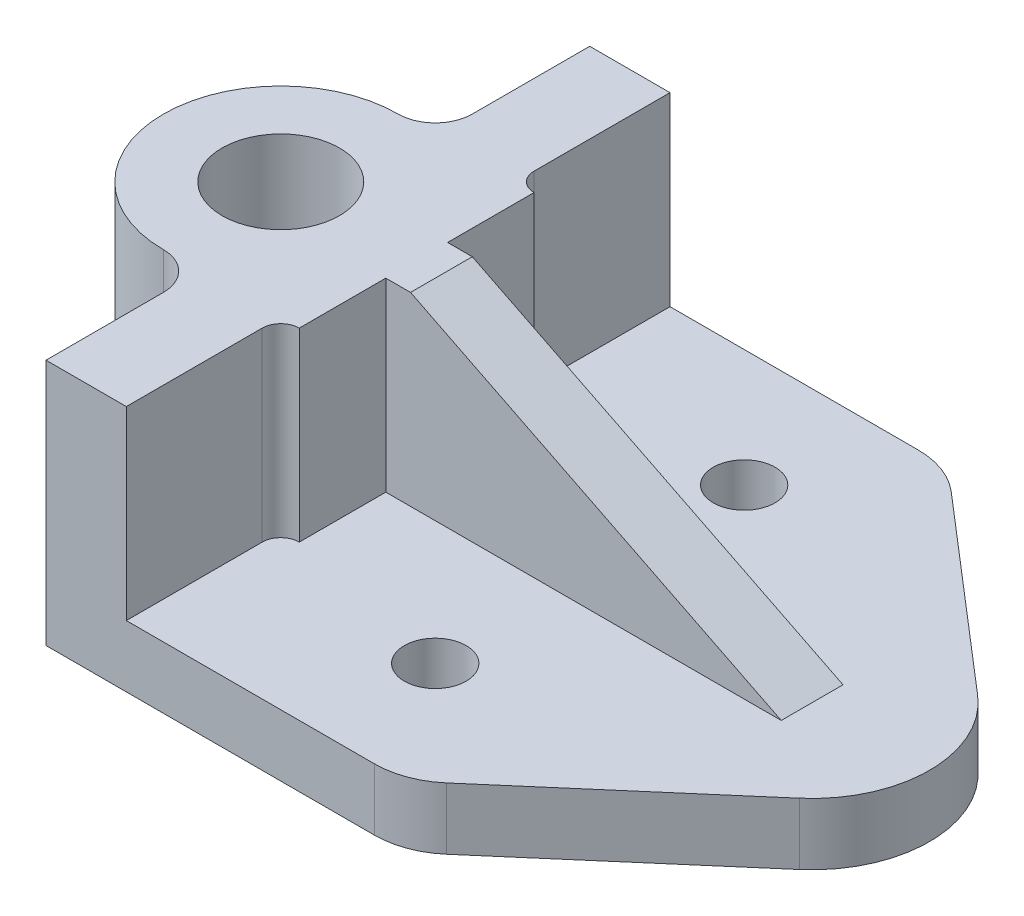
ISO-10303-21;
HEADER;
FILE_DESCRIPTION(('STEP AP214'),'2;1');
FILE_NAME('part.step','',(''),(''),'','','');
FILE_SCHEMA(('AUTOMOTIVE_DESIGN { 1 0 10303 214 1 1 1 1 }'));
ENDSEC;
DATA;
#1=APPLICATION_CONTEXT('core data for automotive mechanical design processes');
#2=APPLICATION_PROTOCOL_DEFINITION('international standard','automotive_design',2000,#1);
#3=PRODUCT_CONTEXT('',#1,'mechanical');
#4=PRODUCT('Part','Part','',(#3));
#5=PRODUCT_RELATED_PRODUCT_CATEGORY('part','',(#4));
#6=PRODUCT_DEFINITION_FORMATION('','',#4);
#7=PRODUCT_DEFINITION_CONTEXT('part definition',#1,'design');
#8=PRODUCT_DEFINITION('design','',#6,#7);
#9=PRODUCT_DEFINITION_SHAPE('','',#8);
#10=(LENGTH_UNIT() NAMED_UNIT(*) SI_UNIT(.MILLI.,.METRE.));
#11=(NAMED_UNIT(*) PLANE_ANGLE_UNIT() SI_UNIT($,.RADIAN.));
#12=(NAMED_UNIT(*) SI_UNIT($,.STERADIAN.) SOLID_ANGLE_UNIT());
#13=UNCERTAINTY_MEASURE_WITH_UNIT(LENGTH_MEASURE(1.E-05),#10,'distance_accuracy_value','');
#14=(GEOMETRIC_REPRESENTATION_CONTEXT(3) GLOBAL_UNCERTAINTY_ASSIGNED_CONTEXT((#13)) GLOBAL_UNIT_ASSIGNED_CONTEXT((#10,
#11,#12)) REPRESENTATION_CONTEXT('',''));
#15=CARTESIAN_POINT('',(0.,0.,0.));
#16=DIRECTION('',(0.,0.,1.));
#17=DIRECTION('',(1.,0.,0.));
#18=AXIS2_PLACEMENT_3D('',#15,#16,#17);
#19=CARTESIAN_POINT('',(-35.5,40.,44.));
#20=DIRECTION('',(-1.,0.,0.));
#21=DIRECTION('',(0.,0.,1.));
#22=AXIS2_PLACEMENT_3D('',#19,#20,#21);
#23=PLANE('',#22);
#24=DIRECTION('',(0.,0.,-1.));
#25=VECTOR('',#24,1.);
#26=CARTESIAN_POINT('',(-35.5,40.,44.));
#27=LINE('',#26,#25);
#28=CARTESIAN_POINT('',(-35.5,40.,44.));
#29=VERTEX_POINT('',#28);
#30=CARTESIAN_POINT('',(-35.5,40.,25.));
#31=VERTEX_POINT('',#30);
#32=EDGE_CURVE('E249',#29,#31,#27,.T.);
#33=ORIENTED_EDGE('',*,*,#32,.T.);
#34=DIRECTION('',(0.,-1.,0.));
#35=VECTOR('',#34,1.);
#36=CARTESIAN_POINT('',(-35.5,0.,25.));
#37=LINE('',#36,#35);
#38=CARTESIAN_POINT('',(-35.5,0.,25.));
#39=VERTEX_POINT('',#38);
#40=EDGE_CURVE('E63',#31,#39,#37,.T.);
#41=ORIENTED_EDGE('',*,*,#40,.T.);
#42=DIRECTION('',(0.,0.,-1.));
#43=VECTOR('',#42,1.);
#44=CARTESIAN_POINT('',(-35.5,0.,44.));
#45=LINE('',#44,#43);
#46=CARTESIAN_POINT('',(-35.5,0.,44.));
#47=VERTEX_POINT('',#46);
#48=EDGE_CURVE('E259',#47,#39,#45,.T.);
#49=ORIENTED_EDGE('',*,*,#48,.F.);
#50=DIRECTION('',(0.,-1.,0.));
#51=VECTOR('',#50,1.);
#52=CARTESIAN_POINT('',(-35.5,40.,44.));
#53=LINE('',#52,#51);
#54=EDGE_CURVE('E261',#29,#47,#53,.T.);
#55=ORIENTED_EDGE('',*,*,#54,.F.);
#56=EDGE_LOOP('',(#33,#41,#49,#55));
#57=FACE_BOUND('',#56,.T.);
#58=ADVANCED_FACE('F43',(#57),#23,.T.);
#59=CARTESIAN_POINT('',(44.5,10.,0.));
#60=DIRECTION('',(0.,1.,0.));
#61=DIRECTION('',(0.,0.,1.));
#62=AXIS2_PLACEMENT_3D('',#59,#60,#61);
#63=PLANE('',#62);
#64=CARTESIAN_POINT('',(8.49999999999999,10.,-25.));
#65=DIRECTION('',(0.,1.,0.));
#66=DIRECTION('',(0.,0.,1.));
#67=AXIS2_PLACEMENT_3D('',#64,#65,#66);
#68=CIRCLE('',#67,5.);
#69=CARTESIAN_POINT('',(8.49999999999999,10.,-20.));
#70=VERTEX_POINT('',#69);
#71=EDGE_CURVE('E308',#70,#70,#68,.T.);
#72=ORIENTED_EDGE('',*,*,#71,.F.);
#73=EDGE_LOOP('',(#72));
#74=FACE_BOUND('',#73,.T.);
#75=CARTESIAN_POINT('',(8.49999999999999,10.,25.));
#76=DIRECTION('',(0.,1.,0.));
#77=DIRECTION('',(0.,0.,1.));
#78=AXIS2_PLACEMENT_3D('',#75,#76,#77);
#79=CIRCLE('',#78,5.);
#80=CARTESIAN_POINT('',(8.49999999999999,10.,30.));
#81=VERTEX_POINT('',#80);
#82=EDGE_CURVE('E399',#81,#81,#79,.T.);
#83=ORIENTED_EDGE('',*,*,#82,.F.);
#84=EDGE_LOOP('',(#83));
#85=FACE_BOUND('',#84,.T.);
#86=DIRECTION('',(0.,0.,1.));
#87=VECTOR('',#86,1.);
#88=CARTESIAN_POINT('',(-22.5,10.,44.));
#89=LINE('',#88,#87);
#90=CARTESIAN_POINT('',(-22.5,10.,-44.));
#91=VERTEX_POINT('',#90);
#92=CARTESIAN_POINT('',(-22.5,10.,-22.));
#93=VERTEX_POINT('',#92);
#94=EDGE_CURVE('E274',#91,#93,#89,.T.);
#95=ORIENTED_EDGE('',*,*,#94,.T.);
#96=CARTESIAN_POINT('',(-19.5,10.,-22.));
#97=DIRECTION('',(0.,1.,0.));
#98=DIRECTION('',(0.,0.,1.));
#99=AXIS2_PLACEMENT_3D('',#96,#97,#98);
#100=CIRCLE('',#99,3.);
#101=CARTESIAN_POINT('',(-19.5,10.,-19.));
#102=VERTEX_POINT('',#101);
#103=EDGE_CURVE('E335',#93,#102,#100,.T.);
#104=ORIENTED_EDGE('',*,*,#103,.T.);
#105=DIRECTION('',(0.,0.,-1.));
#106=VECTOR('',#105,1.);
#107=CARTESIAN_POINT('',(-19.5,10.,19.));
#108=LINE('',#107,#106);
#109=CARTESIAN_POINT('',(-19.5,10.,-5.));
#110=VERTEX_POINT('',#109);
#111=EDGE_CURVE('E233',#110,#102,#108,.T.);
#112=ORIENTED_EDGE('',*,*,#111,.F.);
#113=DIRECTION('',(-1.,0.,0.));
#114=VECTOR('',#113,1.);
#115=CARTESIAN_POINT('',(44.5,10.,-5.));
#116=LINE('',#115,#114);
#117=CARTESIAN_POINT('',(44.5,10.,-5.));
#118=VERTEX_POINT('',#117);
#119=EDGE_CURVE('E217',#118,#110,#116,.T.);
#120=ORIENTED_EDGE('',*,*,#119,.F.);
#121=DIRECTION('',(0.,0.,-1.));
#122=VECTOR('',#121,1.);
#123=CARTESIAN_POINT('',(44.5,10.,5.));
#124=LINE('',#123,#122);
#125=CARTESIAN_POINT('',(44.5,10.,5.00000000000001));
#126=VERTEX_POINT('',#125);
#127=EDGE_CURVE('E218',#126,#118,#124,.T.);
#128=ORIENTED_EDGE('',*,*,#127,.F.);
#129=DIRECTION('',(-1.,0.,0.));
#130=VECTOR('',#129,1.);
#131=CARTESIAN_POINT('',(44.5,10.,5.));
#132=LINE('',#131,#130);
#133=CARTESIAN_POINT('',(-19.5,10.,5.));
#134=VERTEX_POINT('',#133);
#135=EDGE_CURVE('E210',#126,#134,#132,.T.);
#136=ORIENTED_EDGE('',*,*,#135,.T.);
#137=CARTESIAN_POINT('',(-19.5,10.,19.));
#138=VERTEX_POINT('',#137);
#139=EDGE_CURVE('E235',#138,#134,#108,.T.);
#140=ORIENTED_EDGE('',*,*,#139,.F.);
#141=CARTESIAN_POINT('',(-19.5,10.,22.));
#142=DIRECTION('',(0.,1.,0.));
#143=DIRECTION('',(0.,0.,1.));
#144=AXIS2_PLACEMENT_3D('',#141,#142,#143);
#145=CIRCLE('',#144,3.);
#146=CARTESIAN_POINT('',(-22.5,10.,22.));
#147=VERTEX_POINT('',#146);
#148=EDGE_CURVE('E326',#138,#147,#145,.T.);
#149=ORIENTED_EDGE('',*,*,#148,.T.);
#150=CARTESIAN_POINT('',(-22.5,10.,44.));
#151=VERTEX_POINT('',#150);
#152=EDGE_CURVE('E275',#147,#151,#89,.T.);
#153=ORIENTED_EDGE('',*,*,#152,.T.);
#154=DIRECTION('',(1.,0.,0.));
#155=VECTOR('',#154,1.);
#156=CARTESIAN_POINT('',(-22.5,10.,44.));
#157=LINE('',#156,#155);
#158=CARTESIAN_POINT('',(17.6763386057778,10.,44.));
#159=VERTEX_POINT('',#158);
#160=EDGE_CURVE('E276',#151,#159,#157,.T.);
#161=ORIENTED_EDGE('',*,*,#160,.T.);
#162=CARTESIAN_POINT('',(17.6763386057778,10.,31.));
#163=DIRECTION('',(0.,1.,0.));
#164=DIRECTION('',(0.,0.,1.));
#165=AXIS2_PLACEMENT_3D('',#162,#163,#164);
#166=CIRCLE('',#165,13.);
#167=CARTESIAN_POINT('',(26.1561689300687,10.,40.8535515257818));
#168=VERTEX_POINT('',#167);
#169=EDGE_CURVE('E316',#159,#168,#166,.T.);
#170=ORIENTED_EDGE('',*,*,#169,.T.);
#171=DIRECTION('',(0.757965501983215,0.,-0.652294640330068));
#172=VECTOR('',#171,1.);
#173=CARTESIAN_POINT('',(22.5,10.,44.));
#174=LINE('',#173,#172);
#175=CARTESIAN_POINT('',(56.8935981662713,10.,14.4013445376811));
#176=VERTEX_POINT('',#175);
#177=EDGE_CURVE('E277',#168,#176,#174,.T.);
#178=ORIENTED_EDGE('',*,*,#177,.T.);
#179=CARTESIAN_POINT('',(44.5,10.,0.));
#180=DIRECTION('',(0.,1.,0.));
#181=DIRECTION('',(0.,0.,1.));
#182=AXIS2_PLACEMENT_3D('',#179,#180,#181);
#183=CIRCLE('',#182,19.);
#184=CARTESIAN_POINT('',(56.8935981662713,10.,-14.4013445376811));
#185=VERTEX_POINT('',#184);
#186=EDGE_CURVE('E284',#176,#185,#183,.T.);
#187=ORIENTED_EDGE('',*,*,#186,.T.);
#188=DIRECTION('',(-0.757965501983216,0.,-0.652294640330067));
#189=VECTOR('',#188,1.);
#190=CARTESIAN_POINT('',(22.5,10.,-44.));
#191=LINE('',#190,#189);
#192=CARTESIAN_POINT('',(26.1561689300687,10.,-40.8535515257818));
#193=VERTEX_POINT('',#192);
#194=EDGE_CURVE('E285',#185,#193,#191,.T.);
#195=ORIENTED_EDGE('',*,*,#194,.T.);
#196=CARTESIAN_POINT('',(17.6763386057778,10.,-31.));
#197=DIRECTION('',(0.,1.,0.));
#198=DIRECTION('',(0.,0.,1.));
#199=AXIS2_PLACEMENT_3D('',#196,#197,#198);
#200=CIRCLE('',#199,13.);
#201=CARTESIAN_POINT('',(17.6763386057778,10.,-44.));
#202=VERTEX_POINT('',#201);
#203=EDGE_CURVE('E324',#193,#202,#200,.T.);
#204=ORIENTED_EDGE('',*,*,#203,.T.);
#205=DIRECTION('',(-1.,0.,0.));
#206=VECTOR('',#205,1.);
#207=CARTESIAN_POINT('',(-22.5,10.,-44.));
#208=LINE('',#207,#206);
#209=EDGE_CURVE('E269',#202,#91,#208,.T.);
#210=ORIENTED_EDGE('',*,*,#209,.T.);
#211=EDGE_LOOP('',(#95,#104,#112,#120,#128,#136,#140,#149,#153,#161,#170,#178,#187,#195,#204,#210));
#212=FACE_BOUND('',#211,.T.);
#213=ADVANCED_FACE('F393',(#74,#85,#212),#63,.T.);
#214=CARTESIAN_POINT('',(-19.5,0.,0.));
#215=DIRECTION('',(1.,0.,0.));
#216=DIRECTION('',(0.,0.,-1.));
#217=AXIS2_PLACEMENT_3D('',#214,#215,#216);
#218=PLANE('',#217);
#219=ORIENTED_EDGE('',*,*,#139,.T.);
#220=DIRECTION('',(0.,-1.,0.));
#221=VECTOR('',#220,1.);
#222=CARTESIAN_POINT('',(-19.5,40.,5.00000000000001));
#223=LINE('',#222,#221);
#224=CARTESIAN_POINT('',(-19.5,40.,5.00000000000001));
#225=VERTEX_POINT('',#224);
#226=EDGE_CURVE('E400',#225,#134,#223,.T.);
#227=ORIENTED_EDGE('',*,*,#226,.F.);
#228=DIRECTION('',(0.,0.,1.));
#229=VECTOR('',#228,1.);
#230=CARTESIAN_POINT('',(-19.5,40.,19.));
#231=LINE('',#230,#229);
#232=CARTESIAN_POINT('',(-19.5,40.,19.));
#233=VERTEX_POINT('',#232);
#234=EDGE_CURVE('E215',#225,#233,#231,.T.);
#235=ORIENTED_EDGE('',*,*,#234,.T.);
#236=DIRECTION('',(0.,-1.,0.));
#237=VECTOR('',#236,1.);
#238=CARTESIAN_POINT('',(-19.5,40.,19.));
#239=LINE('',#238,#237);
#240=EDGE_CURVE('E226',#233,#138,#239,.T.);
#241=ORIENTED_EDGE('',*,*,#240,.T.);
#242=EDGE_LOOP('',(#219,#227,#235,#241));
#243=FACE_BOUND('',#242,.T.);
#244=ADVANCED_FACE('F435',(#243),#218,.T.);
#245=CARTESIAN_POINT('',(-19.5,40.,-19.));
#246=VERTEX_POINT('',#245);
#247=CARTESIAN_POINT('',(-19.5,40.,-4.99999999999999));
#248=VERTEX_POINT('',#247);
#249=EDGE_CURVE('E238',#246,#248,#231,.T.);
#250=ORIENTED_EDGE('',*,*,#249,.T.);
#251=DIRECTION('',(0.,1.,0.));
#252=VECTOR('',#251,1.);
#253=CARTESIAN_POINT('',(-19.5,40.,-4.99999999999999));
#254=LINE('',#253,#252);
#255=EDGE_CURVE('E216',#110,#248,#254,.T.);
#256=ORIENTED_EDGE('',*,*,#255,.F.);
#257=ORIENTED_EDGE('',*,*,#111,.T.);
#258=DIRECTION('',(0.,1.,0.));
#259=VECTOR('',#258,1.);
#260=CARTESIAN_POINT('',(-19.5,40.,-19.));
#261=LINE('',#260,#259);
#262=EDGE_CURVE('E232',#102,#246,#261,.T.);
#263=ORIENTED_EDGE('',*,*,#262,.T.);
#264=EDGE_LOOP('',(#250,#256,#257,#263));
#265=FACE_BOUND('',#264,.T.);
#266=ADVANCED_FACE('F395',(#265),#218,.T.);
#267=CARTESIAN_POINT('',(-22.5,40.,44.));
#268=DIRECTION('',(1.,0.,0.));
#269=DIRECTION('',(0.,0.,-1.));
#270=AXIS2_PLACEMENT_3D('',#267,#268,#269);
#271=PLANE('',#270);
#272=ORIENTED_EDGE('',*,*,#152,.F.);
#273=DIRECTION('',(0.,-1.,0.));
#274=VECTOR('',#273,1.);
#275=CARTESIAN_POINT('',(-22.5,40.,22.));
#276=LINE('',#275,#274);
#277=CARTESIAN_POINT('',(-22.5,40.,22.));
#278=VERTEX_POINT('',#277);
#279=EDGE_CURVE('E332',#147,#278,#276,.F.);
#280=ORIENTED_EDGE('',*,*,#279,.T.);
#281=DIRECTION('',(0.,0.,1.));
#282=VECTOR('',#281,1.);
#283=CARTESIAN_POINT('',(-22.5,40.,44.));
#284=LINE('',#283,#282);
#285=CARTESIAN_POINT('',(-22.5,40.,44.));
#286=VERTEX_POINT('',#285);
#287=EDGE_CURVE('E246',#278,#286,#284,.T.);
#288=ORIENTED_EDGE('',*,*,#287,.T.);
#289=DIRECTION('',(0.,-1.,0.));
#290=VECTOR('',#289,1.);
#291=CARTESIAN_POINT('',(-22.5,40.,44.));
#292=LINE('',#291,#290);
#293=EDGE_CURVE('E253',#286,#151,#292,.T.);
#294=ORIENTED_EDGE('',*,*,#293,.T.);
#295=EDGE_LOOP('',(#272,#280,#288,#294));
#296=FACE_BOUND('',#295,.T.);
#297=ADVANCED_FACE('F436',(#296),#271,.T.);
#298=CARTESIAN_POINT('',(-22.5,40.,-44.));
#299=VERTEX_POINT('',#298);
#300=CARTESIAN_POINT('',(-22.5,40.,-22.));
#301=VERTEX_POINT('',#300);
#302=EDGE_CURVE('E245',#299,#301,#284,.T.);
#303=ORIENTED_EDGE('',*,*,#302,.T.);
#304=DIRECTION('',(0.,1.,0.));
#305=VECTOR('',#304,1.);
#306=CARTESIAN_POINT('',(-22.5,40.,-22.));
#307=LINE('',#306,#305);
#308=EDGE_CURVE('E327',#301,#93,#307,.F.);
#309=ORIENTED_EDGE('',*,*,#308,.T.);
#310=ORIENTED_EDGE('',*,*,#94,.F.);
#311=DIRECTION('',(0.,-1.,0.));
#312=VECTOR('',#311,1.);
#313=CARTESIAN_POINT('',(-22.5,40.,-44.));
#314=LINE('',#313,#312);
#315=EDGE_CURVE('E260',#299,#91,#314,.T.);
#316=ORIENTED_EDGE('',*,*,#315,.F.);
#317=EDGE_LOOP('',(#303,#309,#310,#316));
#318=FACE_BOUND('',#317,.T.);
#319=ADVANCED_FACE('F385',(#318),#271,.T.);
#320=CARTESIAN_POINT('',(-22.5,10.,-44.));
#321=DIRECTION('',(0.,0.,1.));
#322=DIRECTION('',(1.,0.,0.));
#323=AXIS2_PLACEMENT_3D('',#320,#321,#322);
#324=PLANE('',#323);
#325=ORIENTED_EDGE('',*,*,#209,.F.);
#326=DIRECTION('',(0.,-1.,0.));
#327=VECTOR('',#326,1.);
#328=CARTESIAN_POINT('',(17.6763386057778,10.,-44.));
#329=LINE('',#328,#327);
#330=CARTESIAN_POINT('',(17.6763386057778,0.,-44.));
#331=VERTEX_POINT('',#330);
#332=EDGE_CURVE('E302',#202,#331,#329,.T.);
#333=ORIENTED_EDGE('',*,*,#332,.T.);
#334=DIRECTION('',(-1.,0.,0.));
#335=VECTOR('',#334,1.);
#336=CARTESIAN_POINT('',(-22.5,0.,-44.));
#337=LINE('',#336,#335);
#338=CARTESIAN_POINT('',(-35.5,0.,-44.));
#339=VERTEX_POINT('',#338);
#340=EDGE_CURVE('E263',#331,#339,#337,.T.);
#341=ORIENTED_EDGE('',*,*,#340,.T.);
#342=DIRECTION('',(0.,-1.,0.));
#343=VECTOR('',#342,1.);
#344=CARTESIAN_POINT('',(-35.5,40.,-44.));
#345=LINE('',#344,#343);
#346=CARTESIAN_POINT('',(-35.5,40.,-44.));
#347=VERTEX_POINT('',#346);
#348=EDGE_CURVE('E264',#347,#339,#345,.T.);
#349=ORIENTED_EDGE('',*,*,#348,.F.);
#350=DIRECTION('',(1.,0.,0.));
#351=VECTOR('',#350,1.);
#352=CARTESIAN_POINT('',(-22.5,40.,-44.));
#353=LINE('',#352,#351);
#354=EDGE_CURVE('E255',#347,#299,#353,.T.);
#355=ORIENTED_EDGE('',*,*,#354,.T.);
#356=ORIENTED_EDGE('',*,*,#315,.T.);
#357=EDGE_LOOP('',(#325,#333,#341,#349,#355,#356));
#358=FACE_BOUND('',#357,.T.);
#359=ADVANCED_FACE('F380',(#358),#324,.F.);
#360=CARTESIAN_POINT('',(-22.5,10.,44.));
#361=DIRECTION('',(0.,0.,-1.));
#362=DIRECTION('',(-1.,0.,0.));
#363=AXIS2_PLACEMENT_3D('',#360,#361,#362);
#364=PLANE('',#363);
#365=DIRECTION('',(1.,0.,0.));
#366=VECTOR('',#365,1.);
#367=CARTESIAN_POINT('',(-22.5,0.,44.));
#368=LINE('',#367,#366);
#369=CARTESIAN_POINT('',(17.6763386057778,0.,44.));
#370=VERTEX_POINT('',#369);
#371=EDGE_CURVE('E289',#47,#370,#368,.T.);
#372=ORIENTED_EDGE('',*,*,#371,.T.);
#373=DIRECTION('',(0.,-1.,0.));
#374=VECTOR('',#373,1.);
#375=CARTESIAN_POINT('',(17.6763386057778,10.,44.));
#376=LINE('',#375,#374);
#377=EDGE_CURVE('E328',#370,#159,#376,.F.);
#378=ORIENTED_EDGE('',*,*,#377,.T.);
#379=ORIENTED_EDGE('',*,*,#160,.F.);
#380=ORIENTED_EDGE('',*,*,#293,.F.);
#381=DIRECTION('',(-1.,0.,0.));
#382=VECTOR('',#381,1.);
#383=CARTESIAN_POINT('',(-22.5,40.,44.));
#384=LINE('',#383,#382);
#385=EDGE_CURVE('E244',#286,#29,#384,.T.);
#386=ORIENTED_EDGE('',*,*,#385,.T.);
#387=ORIENTED_EDGE('',*,*,#54,.T.);
#388=EDGE_LOOP('',(#372,#378,#379,#380,#386,#387));
#389=FACE_BOUND('',#388,.T.);
#390=ADVANCED_FACE('F455',(#389),#364,.F.);
#391=CARTESIAN_POINT('',(22.5,10.,44.));
#392=DIRECTION('',(-0.652294640330068,0.,-0.757965501983215));
#393=DIRECTION('',(-0.757965501983215,0.,0.652294640330068));
#394=AXIS2_PLACEMENT_3D('',#391,#392,#393);
#395=PLANE('',#394);
#396=ORIENTED_EDGE('',*,*,#177,.F.);
#397=DIRECTION('',(0.,-1.,0.));
#398=VECTOR('',#397,1.);
#399=CARTESIAN_POINT('',(26.1561689300687,10.,40.8535515257818));
#400=LINE('',#399,#398);
#401=CARTESIAN_POINT('',(26.1561689300687,0.,40.8535515257818));
#402=VERTEX_POINT('',#401);
#403=EDGE_CURVE('E325',#168,#402,#400,.T.);
#404=ORIENTED_EDGE('',*,*,#403,.T.);
#405=DIRECTION('',(0.757965501983215,0.,-0.652294640330068));
#406=VECTOR('',#405,1.);
#407=CARTESIAN_POINT('',(22.5,0.,44.));
#408=LINE('',#407,#406);
#409=CARTESIAN_POINT('',(56.8935981662713,0.,14.4013445376811));
#410=VERTEX_POINT('',#409);
#411=EDGE_CURVE('E291',#402,#410,#408,.T.);
#412=ORIENTED_EDGE('',*,*,#411,.T.);
#413=DIRECTION('',(0.,-1.,0.));
#414=VECTOR('',#413,1.);
#415=CARTESIAN_POINT('',(56.8935981662713,10.,14.4013445376811));
#416=LINE('',#415,#414);
#417=EDGE_CURVE('E301',#176,#410,#416,.T.);
#418=ORIENTED_EDGE('',*,*,#417,.F.);
#419=EDGE_LOOP('',(#396,#404,#412,#418));
#420=FACE_BOUND('',#419,.T.);
#421=ADVANCED_FACE('F446',(#420),#395,.F.);
#422=CARTESIAN_POINT('',(44.5,10.,0.));
#423=DIRECTION('',(0.,-1.,0.));
#424=DIRECTION('',(0.,0.,-1.));
#425=AXIS2_PLACEMENT_3D('',#422,#423,#424);
#426=CYLINDRICAL_SURFACE('',#425,19.);
#427=CARTESIAN_POINT('',(44.5,0.,0.));
#428=DIRECTION('',(0.,1.,0.));
#429=DIRECTION('',(0.,0.,1.));
#430=AXIS2_PLACEMENT_3D('',#427,#428,#429);
#431=CIRCLE('',#430,19.);
#432=CARTESIAN_POINT('',(56.8935981662713,0.,-14.4013445376811));
#433=VERTEX_POINT('',#432);
#434=EDGE_CURVE('E294',#410,#433,#431,.T.);
#435=ORIENTED_EDGE('',*,*,#434,.T.);
#436=DIRECTION('',(0.,-1.,0.));
#437=VECTOR('',#436,1.);
#438=CARTESIAN_POINT('',(56.8935981662713,10.,-14.4013445376811));
#439=LINE('',#438,#437);
#440=EDGE_CURVE('E290',#185,#433,#439,.T.);
#441=ORIENTED_EDGE('',*,*,#440,.F.);
#442=ORIENTED_EDGE('',*,*,#186,.F.);
#443=ORIENTED_EDGE('',*,*,#417,.T.);
#444=EDGE_LOOP('',(#435,#441,#442,#443));
#445=FACE_BOUND('',#444,.T.);
#446=ADVANCED_FACE('F444',(#445),#426,.T.);
#447=CARTESIAN_POINT('',(22.5,10.,-44.));
#448=DIRECTION('',(-0.652294640330067,0.,0.757965501983216));
#449=DIRECTION('',(0.757965501983216,0.,0.652294640330067));
#450=AXIS2_PLACEMENT_3D('',#447,#448,#449);
#451=PLANE('',#450);
#452=DIRECTION('',(-0.757965501983216,0.,-0.652294640330067));
#453=VECTOR('',#452,1.);
#454=CARTESIAN_POINT('',(22.5,0.,-44.));
#455=LINE('',#454,#453);
#456=CARTESIAN_POINT('',(26.1561689300687,0.,-40.8535515257818));
#457=VERTEX_POINT('',#456);
#458=EDGE_CURVE('E271',#433,#457,#455,.T.);
#459=ORIENTED_EDGE('',*,*,#458,.T.);
#460=DIRECTION('',(0.,-1.,0.));
#461=VECTOR('',#460,1.);
#462=CARTESIAN_POINT('',(26.1561689300687,10.,-40.8535515257818));
#463=LINE('',#462,#461);
#464=EDGE_CURVE('E320',#457,#193,#463,.F.);
#465=ORIENTED_EDGE('',*,*,#464,.T.);
#466=ORIENTED_EDGE('',*,*,#194,.F.);
#467=ORIENTED_EDGE('',*,*,#440,.T.);
#468=EDGE_LOOP('',(#459,#465,#466,#467));
#469=FACE_BOUND('',#468,.T.);
#470=ADVANCED_FACE('F441',(#469),#451,.F.);
#471=CARTESIAN_POINT('',(44.5,0.,0.));
#472=DIRECTION('',(0.,1.,0.));
#473=DIRECTION('',(0.,0.,1.));
#474=AXIS2_PLACEMENT_3D('',#471,#472,#473);
#475=PLANE('',#474);
#476=CARTESIAN_POINT('',(-41.5,0.,0.));
#477=DIRECTION('',(0.,1.,0.));
#478=DIRECTION('',(0.,0.,1.));
#479=AXIS2_PLACEMENT_3D('',#476,#477,#478);
#480=CIRCLE('',#479,9.5);
#481=CARTESIAN_POINT('',(-41.5,0.,9.50000000000001));
#482=VERTEX_POINT('',#481);
#483=EDGE_CURVE('E362',#482,#482,#480,.T.);
#484=ORIENTED_EDGE('',*,*,#483,.T.);
#485=EDGE_LOOP('',(#484));
#486=FACE_BOUND('',#485,.T.);
#487=CARTESIAN_POINT('',(8.49999999999999,0.,-25.));
#488=DIRECTION('',(0.,1.,0.));
#489=DIRECTION('',(0.,0.,1.));
#490=AXIS2_PLACEMENT_3D('',#487,#488,#489);
#491=CIRCLE('',#490,5.);
#492=CARTESIAN_POINT('',(8.49999999999999,0.,-20.));
#493=VERTEX_POINT('',#492);
#494=EDGE_CURVE('E206',#493,#493,#491,.T.);
#495=ORIENTED_EDGE('',*,*,#494,.T.);
#496=EDGE_LOOP('',(#495));
#497=FACE_BOUND('',#496,.T.);
#498=CARTESIAN_POINT('',(8.49999999999999,0.,25.));
#499=DIRECTION('',(0.,1.,0.));
#500=DIRECTION('',(0.,0.,1.));
#501=AXIS2_PLACEMENT_3D('',#498,#499,#500);
#502=CIRCLE('',#501,5.);
#503=CARTESIAN_POINT('',(8.49999999999999,0.,30.));
#504=VERTEX_POINT('',#503);
#505=EDGE_CURVE('E304',#504,#504,#502,.T.);
#506=ORIENTED_EDGE('',*,*,#505,.T.);
#507=EDGE_LOOP('',(#506));
#508=FACE_BOUND('',#507,.T.);
#509=ORIENTED_EDGE('',*,*,#340,.F.);
#510=CARTESIAN_POINT('',(17.6763386057778,0.,-31.));
#511=DIRECTION('',(0.,1.,0.));
#512=DIRECTION('',(0.,0.,1.));
#513=AXIS2_PLACEMENT_3D('',#510,#511,#512);
#514=CIRCLE('',#513,13.);
#515=EDGE_CURVE('E314',#331,#457,#514,.F.);
#516=ORIENTED_EDGE('',*,*,#515,.T.);
#517=ORIENTED_EDGE('',*,*,#458,.F.);
#518=ORIENTED_EDGE('',*,*,#434,.F.);
#519=ORIENTED_EDGE('',*,*,#411,.F.);
#520=CARTESIAN_POINT('',(17.6763386057778,0.,31.));
#521=DIRECTION('',(0.,1.,0.));
#522=DIRECTION('',(0.,0.,1.));
#523=AXIS2_PLACEMENT_3D('',#520,#521,#522);
#524=CIRCLE('',#523,13.);
#525=EDGE_CURVE('E312',#402,#370,#524,.F.);
#526=ORIENTED_EDGE('',*,*,#525,.T.);
#527=ORIENTED_EDGE('',*,*,#371,.F.);
#528=ORIENTED_EDGE('',*,*,#48,.T.);
#529=CARTESIAN_POINT('',(-41.5,0.,25.));
#530=DIRECTION('',(0.,1.,0.));
#531=DIRECTION('',(0.,0.,1.));
#532=AXIS2_PLACEMENT_3D('',#529,#530,#531);
#533=CIRCLE('',#532,6.);
#534=CARTESIAN_POINT('',(-41.5,0.,19.));
#535=VERTEX_POINT('',#534);
#536=EDGE_CURVE('E11',#39,#535,#533,.T.);
#537=ORIENTED_EDGE('',*,*,#536,.T.);
#538=CARTESIAN_POINT('',(-41.5,0.,0.));
#539=DIRECTION('',(0.,1.,0.));
#540=DIRECTION('',(0.,0.,1.));
#541=AXIS2_PLACEMENT_3D('',#538,#539,#540);
#542=CIRCLE('',#541,19.);
#543=CARTESIAN_POINT('',(-41.5,0.,-19.));
#544=VERTEX_POINT('',#543);
#545=EDGE_CURVE('E364',#535,#544,#542,.F.);
#546=ORIENTED_EDGE('',*,*,#545,.T.);
#547=CARTESIAN_POINT('',(-41.5,0.,-25.));
#548=DIRECTION('',(0.,1.,0.));
#549=DIRECTION('',(0.,0.,1.));
#550=AXIS2_PLACEMENT_3D('',#547,#548,#549);
#551=CIRCLE('',#550,6.);
#552=CARTESIAN_POINT('',(-35.5,0.,-25.));
#553=VERTEX_POINT('',#552);
#554=EDGE_CURVE('E350',#544,#553,#551,.T.);
#555=ORIENTED_EDGE('',*,*,#554,.T.);
#556=EDGE_CURVE('E241',#553,#339,#45,.T.);
#557=ORIENTED_EDGE('',*,*,#556,.T.);
#558=EDGE_LOOP('',(#509,#516,#517,#518,#519,#526,#527,#528,#537,#546,#555,#557));
#559=FACE_BOUND('',#558,.T.);
#560=ADVANCED_FACE('F371',(#486,#497,#508,#559),#475,.F.);
#561=ORIENTED_EDGE('',*,*,#556,.F.);
#562=DIRECTION('',(0.,-1.,0.));
#563=VECTOR('',#562,1.);
#564=CARTESIAN_POINT('',(-35.5,40.,-25.));
#565=LINE('',#564,#563);
#566=CARTESIAN_POINT('',(-35.5,40.,-25.));
#567=VERTEX_POINT('',#566);
#568=EDGE_CURVE('E348',#553,#567,#565,.F.);
#569=ORIENTED_EDGE('',*,*,#568,.T.);
#570=EDGE_CURVE('E248',#567,#347,#27,.T.);
#571=ORIENTED_EDGE('',*,*,#570,.T.);
#572=ORIENTED_EDGE('',*,*,#348,.T.);
#573=EDGE_LOOP('',(#561,#569,#571,#572));
#574=FACE_BOUND('',#573,.T.);
#575=ADVANCED_FACE('F373',(#574),#23,.T.);
#576=CARTESIAN_POINT('',(0.,40.,0.));
#577=DIRECTION('',(0.,1.,0.));
#578=DIRECTION('',(0.,0.,1.));
#579=AXIS2_PLACEMENT_3D('',#576,#577,#578);
#580=PLANE('',#579);
#581=CARTESIAN_POINT('',(-41.5,40.,0.));
#582=DIRECTION('',(0.,1.,0.));
#583=DIRECTION('',(0.,0.,1.));
#584=AXIS2_PLACEMENT_3D('',#581,#582,#583);
#585=CIRCLE('',#584,9.5);
#586=CARTESIAN_POINT('',(-41.5,40.,9.50000000000001));
#587=VERTEX_POINT('',#586);
#588=EDGE_CURVE('E410',#587,#587,#585,.T.);
#589=ORIENTED_EDGE('',*,*,#588,.F.);
#590=EDGE_LOOP('',(#589));
#591=FACE_BOUND('',#590,.T.);
#592=ORIENTED_EDGE('',*,*,#570,.F.);
#593=CARTESIAN_POINT('',(-41.5,40.,-25.));
#594=DIRECTION('',(0.,1.,0.));
#595=DIRECTION('',(0.,0.,1.));
#596=AXIS2_PLACEMENT_3D('',#593,#594,#595);
#597=CIRCLE('',#596,6.);
#598=CARTESIAN_POINT('',(-41.5,40.,-19.));
#599=VERTEX_POINT('',#598);
#600=EDGE_CURVE('E353',#567,#599,#597,.F.);
#601=ORIENTED_EDGE('',*,*,#600,.T.);
#602=CARTESIAN_POINT('',(-41.5,40.,0.));
#603=DIRECTION('',(0.,1.,0.));
#604=DIRECTION('',(0.,0.,1.));
#605=AXIS2_PLACEMENT_3D('',#602,#603,#604);
#606=CIRCLE('',#605,19.);
#607=CARTESIAN_POINT('',(-41.5,40.,19.));
#608=VERTEX_POINT('',#607);
#609=EDGE_CURVE('E352',#599,#608,#606,.T.);
#610=ORIENTED_EDGE('',*,*,#609,.T.);
#611=CARTESIAN_POINT('',(-41.5,40.,25.));
#612=DIRECTION('',(0.,1.,0.));
#613=DIRECTION('',(0.,0.,1.));
#614=AXIS2_PLACEMENT_3D('',#611,#612,#613);
#615=CIRCLE('',#614,6.);
#616=EDGE_CURVE('E51',#608,#31,#615,.F.);
#617=ORIENTED_EDGE('',*,*,#616,.T.);
#618=ORIENTED_EDGE('',*,*,#32,.F.);
#619=ORIENTED_EDGE('',*,*,#385,.F.);
#620=ORIENTED_EDGE('',*,*,#287,.F.);
#621=CARTESIAN_POINT('',(-19.5,40.,22.));
#622=DIRECTION('',(0.,1.,0.));
#623=DIRECTION('',(0.,0.,1.));
#624=AXIS2_PLACEMENT_3D('',#621,#622,#623);
#625=CIRCLE('',#624,3.);
#626=EDGE_CURVE('E336',#278,#233,#625,.F.);
#627=ORIENTED_EDGE('',*,*,#626,.T.);
#628=ORIENTED_EDGE('',*,*,#234,.F.);
#629=DIRECTION('',(-1.,0.,0.));
#630=VECTOR('',#629,1.);
#631=CARTESIAN_POINT('',(44.5,40.,5.00000000000001));
#632=LINE('',#631,#630);
#633=CARTESIAN_POINT('',(-15.5,40.,5.));
#634=VERTEX_POINT('',#633);
#635=EDGE_CURVE('E204',#634,#225,#632,.T.);
#636=ORIENTED_EDGE('',*,*,#635,.F.);
#637=DIRECTION('',(0.,0.,1.));
#638=VECTOR('',#637,1.);
#639=CARTESIAN_POINT('',(-15.5,40.,-59.));
#640=LINE('',#639,#638);
#641=CARTESIAN_POINT('',(-15.5,40.,-5.));
#642=VERTEX_POINT('',#641);
#643=EDGE_CURVE('E194',#642,#634,#640,.T.);
#644=ORIENTED_EDGE('',*,*,#643,.F.);
#645=DIRECTION('',(-1.,0.,0.));
#646=VECTOR('',#645,1.);
#647=CARTESIAN_POINT('',(44.5,40.,-4.99999999999999));
#648=LINE('',#647,#646);
#649=EDGE_CURVE('E212',#642,#248,#648,.T.);
#650=ORIENTED_EDGE('',*,*,#649,.T.);
#651=ORIENTED_EDGE('',*,*,#249,.F.);
#652=CARTESIAN_POINT('',(-19.5,40.,-22.));
#653=DIRECTION('',(0.,1.,0.));
#654=DIRECTION('',(0.,0.,1.));
#655=AXIS2_PLACEMENT_3D('',#652,#653,#654);
#656=CIRCLE('',#655,3.);
#657=EDGE_CURVE('E337',#246,#301,#656,.F.);
#658=ORIENTED_EDGE('',*,*,#657,.T.);
#659=ORIENTED_EDGE('',*,*,#302,.F.);
#660=ORIENTED_EDGE('',*,*,#354,.F.);
#661=EDGE_LOOP('',(#592,#601,#610,#617,#618,#619,#620,#627,#628,#636,#644,#650,#651,#658,#659,#660));
#662=FACE_BOUND('',#661,.T.);
#663=ADVANCED_FACE('F214',(#591,#662),#580,.T.);
#664=CARTESIAN_POINT('',(44.5,40.,5.00000000000001));
#665=DIRECTION('',(0.,0.,-1.));
#666=DIRECTION('',(0.,1.,0.));
#667=AXIS2_PLACEMENT_3D('',#664,#665,#666);
#668=PLANE('',#667);
#669=ORIENTED_EDGE('',*,*,#135,.F.);
#670=DIRECTION('',(0.894427190999916,-0.447213595499958,0.));
#671=VECTOR('',#670,1.);
#672=CARTESIAN_POINT('',(44.5,10.,5.));
#673=LINE('',#672,#671);
#674=EDGE_CURVE('E193',#634,#126,#673,.T.);
#675=ORIENTED_EDGE('',*,*,#674,.F.);
#676=ORIENTED_EDGE('',*,*,#635,.T.);
#677=ORIENTED_EDGE('',*,*,#226,.T.);
#678=EDGE_LOOP('',(#669,#675,#676,#677));
#679=FACE_BOUND('',#678,.T.);
#680=ADVANCED_FACE('F201',(#679),#668,.F.);
#681=CARTESIAN_POINT('',(44.5,40.,-4.99999999999999));
#682=DIRECTION('',(0.,0.,1.));
#683=DIRECTION('',(0.,-1.,0.));
#684=AXIS2_PLACEMENT_3D('',#681,#682,#683);
#685=PLANE('',#684);
#686=ORIENTED_EDGE('',*,*,#649,.F.);
#687=DIRECTION('',(0.894427190999916,-0.447213595499958,0.));
#688=VECTOR('',#687,1.);
#689=CARTESIAN_POINT('',(32.5,16.,-5.));
#690=LINE('',#689,#688);
#691=EDGE_CURVE('E199',#642,#118,#690,.T.);
#692=ORIENTED_EDGE('',*,*,#691,.T.);
#693=ORIENTED_EDGE('',*,*,#119,.T.);
#694=ORIENTED_EDGE('',*,*,#255,.T.);
#695=EDGE_LOOP('',(#686,#692,#693,#694));
#696=FACE_BOUND('',#695,.T.);
#697=ADVANCED_FACE('F422',(#696),#685,.F.);
#698=CARTESIAN_POINT('',(44.5,10.,-59.));
#699=DIRECTION('',(-0.447213595499958,-0.894427190999916,0.));
#700=DIRECTION('',(0.894427190999916,-0.447213595499958,0.));
#701=AXIS2_PLACEMENT_3D('',#698,#699,#700);
#702=PLANE('',#701);
#703=ORIENTED_EDGE('',*,*,#643,.T.);
#704=ORIENTED_EDGE('',*,*,#674,.T.);
#705=ORIENTED_EDGE('',*,*,#127,.T.);
#706=ORIENTED_EDGE('',*,*,#691,.F.);
#707=EDGE_LOOP('',(#703,#704,#705,#706));
#708=FACE_BOUND('',#707,.T.);
#709=ADVANCED_FACE('F195',(#708),#702,.F.);
#710=CARTESIAN_POINT('',(8.49999999999999,-54.,25.));
#711=DIRECTION('',(0.,1.,0.));
#712=DIRECTION('',(0.,0.,1.));
#713=AXIS2_PLACEMENT_3D('',#710,#711,#712);
#714=CYLINDRICAL_SURFACE('',#713,5.);
#715=ORIENTED_EDGE('',*,*,#82,.T.);
#716=EDGE_LOOP('',(#715));
#717=FACE_BOUND('',#716,.T.);
#718=ORIENTED_EDGE('',*,*,#505,.F.);
#719=EDGE_LOOP('',(#718));
#720=FACE_BOUND('',#719,.T.);
#721=ADVANCED_FACE('F492',(#717,#720),#714,.F.);
#722=CARTESIAN_POINT('',(8.49999999999999,-54.,-25.));
#723=DIRECTION('',(0.,1.,0.));
#724=DIRECTION('',(0.,0.,1.));
#725=AXIS2_PLACEMENT_3D('',#722,#723,#724);
#726=CYLINDRICAL_SURFACE('',#725,5.);
#727=ORIENTED_EDGE('',*,*,#71,.T.);
#728=EDGE_LOOP('',(#727));
#729=FACE_BOUND('',#728,.T.);
#730=ORIENTED_EDGE('',*,*,#494,.F.);
#731=EDGE_LOOP('',(#730));
#732=FACE_BOUND('',#731,.T.);
#733=ADVANCED_FACE('F560',(#729,#732),#726,.F.);
#734=CARTESIAN_POINT('',(-41.5,-53.7401153701776,0.));
#735=DIRECTION('',(0.,1.,0.));
#736=DIRECTION('',(0.,0.,1.));
#737=AXIS2_PLACEMENT_3D('',#734,#735,#736);
#738=CYLINDRICAL_SURFACE('',#737,19.);
#739=ORIENTED_EDGE('',*,*,#609,.F.);
#740=DIRECTION('',(0.,1.,0.));
#741=VECTOR('',#740,1.);
#742=CARTESIAN_POINT('',(-41.5,-53.7401153701776,-19.));
#743=LINE('',#742,#741);
#744=EDGE_CURVE('E345',#599,#544,#743,.F.);
#745=ORIENTED_EDGE('',*,*,#744,.T.);
#746=ORIENTED_EDGE('',*,*,#545,.F.);
#747=DIRECTION('',(0.,1.,0.));
#748=VECTOR('',#747,1.);
#749=CARTESIAN_POINT('',(-41.5,-53.7401153701776,19.));
#750=LINE('',#749,#748);
#751=EDGE_CURVE('E338',#535,#608,#750,.T.);
#752=ORIENTED_EDGE('',*,*,#751,.T.);
#753=EDGE_LOOP('',(#739,#745,#746,#752));
#754=FACE_BOUND('',#753,.T.);
#755=ADVANCED_FACE('F359',(#754),#738,.T.);
#756=CARTESIAN_POINT('',(-41.5,-24.,0.));
#757=DIRECTION('',(0.,1.,0.));
#758=DIRECTION('',(0.,0.,1.));
#759=AXIS2_PLACEMENT_3D('',#756,#757,#758);
#760=CYLINDRICAL_SURFACE('',#759,9.5);
#761=ORIENTED_EDGE('',*,*,#588,.T.);
#762=EDGE_LOOP('',(#761));
#763=FACE_BOUND('',#762,.T.);
#764=ORIENTED_EDGE('',*,*,#483,.F.);
#765=EDGE_LOOP('',(#764));
#766=FACE_BOUND('',#765,.T.);
#767=ADVANCED_FACE('F414',(#763,#766),#760,.F.);
#768=CARTESIAN_POINT('',(17.6763386057778,10.,-31.));
#769=DIRECTION('',(0.,-1.,0.));
#770=DIRECTION('',(0.,0.,-1.));
#771=AXIS2_PLACEMENT_3D('',#768,#769,#770);
#772=CYLINDRICAL_SURFACE('',#771,13.);
#773=ORIENTED_EDGE('',*,*,#203,.F.);
#774=ORIENTED_EDGE('',*,*,#464,.F.);
#775=ORIENTED_EDGE('',*,*,#515,.F.);
#776=ORIENTED_EDGE('',*,*,#332,.F.);
#777=EDGE_LOOP('',(#773,#774,#775,#776));
#778=FACE_BOUND('',#777,.T.);
#779=ADVANCED_FACE('F456',(#778),#772,.T.);
#780=CARTESIAN_POINT('',(17.6763386057778,10.,31.));
#781=DIRECTION('',(0.,-1.,0.));
#782=DIRECTION('',(0.,0.,-1.));
#783=AXIS2_PLACEMENT_3D('',#780,#781,#782);
#784=CYLINDRICAL_SURFACE('',#783,13.);
#785=ORIENTED_EDGE('',*,*,#169,.F.);
#786=ORIENTED_EDGE('',*,*,#377,.F.);
#787=ORIENTED_EDGE('',*,*,#525,.F.);
#788=ORIENTED_EDGE('',*,*,#403,.F.);
#789=EDGE_LOOP('',(#785,#786,#787,#788));
#790=FACE_BOUND('',#789,.T.);
#791=ADVANCED_FACE('F461',(#790),#784,.T.);
#792=CARTESIAN_POINT('',(-19.5,40.,-22.));
#793=DIRECTION('',(0.,1.,0.));
#794=DIRECTION('',(0.,0.,1.));
#795=AXIS2_PLACEMENT_3D('',#792,#793,#794);
#796=CYLINDRICAL_SURFACE('',#795,3.);
#797=ORIENTED_EDGE('',*,*,#103,.F.);
#798=ORIENTED_EDGE('',*,*,#308,.F.);
#799=ORIENTED_EDGE('',*,*,#657,.F.);
#800=ORIENTED_EDGE('',*,*,#262,.F.);
#801=EDGE_LOOP('',(#797,#798,#799,#800));
#802=FACE_BOUND('',#801,.T.);
#803=ADVANCED_FACE('F389',(#802),#796,.F.);
#804=CARTESIAN_POINT('',(-19.5,40.,22.));
#805=DIRECTION('',(0.,-1.,0.));
#806=DIRECTION('',(0.,0.,-1.));
#807=AXIS2_PLACEMENT_3D('',#804,#805,#806);
#808=CYLINDRICAL_SURFACE('',#807,3.);
#809=ORIENTED_EDGE('',*,*,#626,.F.);
#810=ORIENTED_EDGE('',*,*,#279,.F.);
#811=ORIENTED_EDGE('',*,*,#148,.F.);
#812=ORIENTED_EDGE('',*,*,#240,.F.);
#813=EDGE_LOOP('',(#809,#810,#811,#812));
#814=FACE_BOUND('',#813,.T.);
#815=ADVANCED_FACE('F468',(#814),#808,.F.);
#816=CARTESIAN_POINT('',(-41.5,-53.7401153701776,-25.));
#817=DIRECTION('',(0.,1.,0.));
#818=DIRECTION('',(0.,0.,1.));
#819=AXIS2_PLACEMENT_3D('',#816,#817,#818);
#820=CYLINDRICAL_SURFACE('',#819,6.);
#821=ORIENTED_EDGE('',*,*,#600,.F.);
#822=ORIENTED_EDGE('',*,*,#568,.F.);
#823=ORIENTED_EDGE('',*,*,#554,.F.);
#824=ORIENTED_EDGE('',*,*,#744,.F.);
#825=EDGE_LOOP('',(#821,#822,#823,#824));
#826=FACE_BOUND('',#825,.T.);
#827=ADVANCED_FACE('F370',(#826),#820,.F.);
#828=CARTESIAN_POINT('',(-41.5,-53.7401153701776,25.));
#829=DIRECTION('',(0.,1.,0.));
#830=DIRECTION('',(0.,0.,1.));
#831=AXIS2_PLACEMENT_3D('',#828,#829,#830);
#832=CYLINDRICAL_SURFACE('',#831,6.);
#833=ORIENTED_EDGE('',*,*,#536,.F.);
#834=ORIENTED_EDGE('',*,*,#40,.F.);
#835=ORIENTED_EDGE('',*,*,#616,.F.);
#836=ORIENTED_EDGE('',*,*,#751,.F.);
#837=EDGE_LOOP('',(#833,#834,#835,#836));
#838=FACE_BOUND('',#837,.T.);
#839=ADVANCED_FACE('F44',(#838),#832,.F.);
#840=CLOSED_SHELL('',(#58,#213,#244,#266,#297,#319,#359,#390,#421,#446,#470,#560,#575,#663,#680,
#697,#709,#721,#733,#755,#767,#779,#791,#803,#815,#827,#839));
#841=MANIFOLD_SOLID_BREP('B2',#840);
#842=ADVANCED_BREP_SHAPE_REPRESENTATION('',(#18,#841),#14);
#843=SHAPE_DEFINITION_REPRESENTATION(#9,#842);
ENDSEC;
END-ISO-10303-21;
